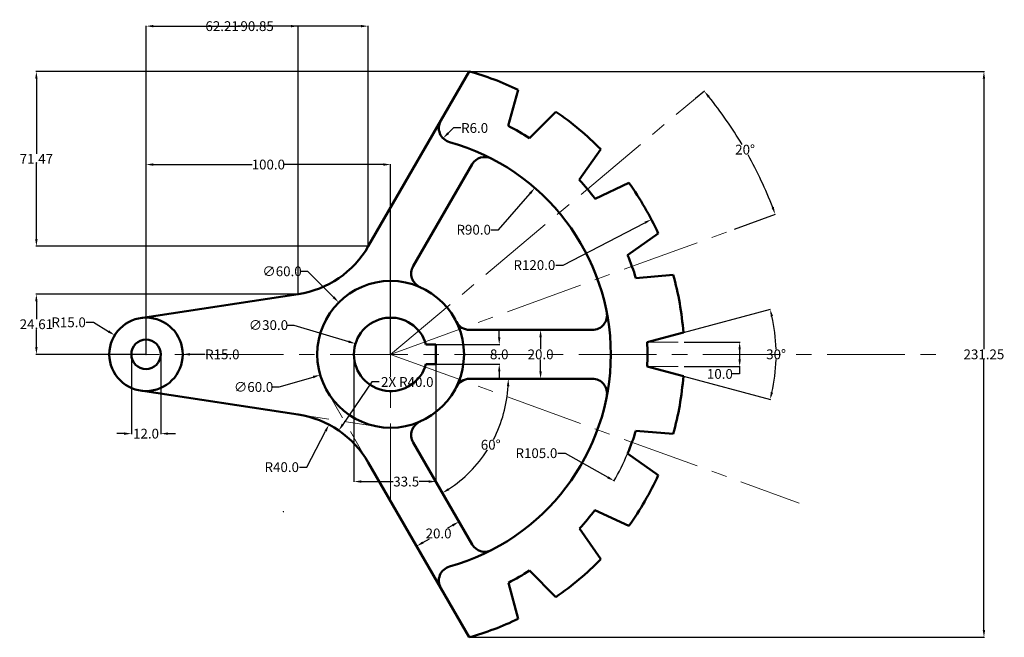
# Model space of a CAD drawing. Units: inches. Extents: x 327 to 730, y 258 to 510.
import ezdxf

# ---------------------------------------------------------------- set-up
doc = ezdxf.new("R2010")
doc.units = ezdxf.units.IN
doc.header["$MEASUREMENT"] = 0
doc.linetypes.add('CENTER', pattern=[50.8, 31.75, -6.35, 6.35, -6.35])
doc.linetypes.add('DASHED', pattern=[19.05, 12.7, -6.35])
for name, color, linetype, lineweight in [('M-CNTR', 4, 'CENTER', 18), ('M-CONS', 8, 'DASHED', 13), ('M-DIMS', 2, 'Continuous', 25), ('M-OUTL', 7, 'Continuous', 50)]:
    doc.layers.add(name, color=color, linetype=linetype, lineweight=lineweight)
doc.styles.get("Standard").update_dxf_attribs({"font": 'arial.ttf'})
doc.dimstyles.get("Standard").update_dxf_attribs({"dimtxt": 4, "dimasz": 3, "dimexe": 0.18, "dimexo": 0.0625, "dimgap": 0.09, "dimtad": 0, "dimtih": 1, "dimtoh": 1, "dimdec": 1, "dimzin": 0, "dimdsep": 46, "dimtxsty": 'Standard', "dimcen": 0.09, "dimadec": 0, "dimazin": 0, "dimtfac": 1, "dimtdec": 1, "dimtofl": 0, "dimtmove": 0, "dimatfit": 3, "dimfxl": 1, "dimtolj": 1, "dimtzin": 0, "dimarcsym": 0})

# ---------------------------------------------------------------- blocks, each defined once
blk = doc.blocks.new('*D1')
at = {"layer": 'Defpoints', "color": 0, "transparency": 16777216}
for p in [(463.65, 373.45), (497.15, 373.45), (497.15, 321.47)]:
    blk.add_point(p, dxfattribs=at)
at = {"layer": 'M-DIMS', "color": 0, "lineweight": -2, "transparency": 16777216}
for p, q in [((463.65, 373.39), (463.65, 321.29)), ((497.15, 373.39), (497.15, 321.29)), ((466.65, 321.47), (479.73, 321.47)), ((494.15, 321.47), (490.33, 321.47))]:
    blk.add_line(p, q, dxfattribs=at)
at = {"layer": 'M-DIMS', "color": 0, "transparency": 16777216}
for points in [[(466.65, 321.97), (466.65, 320.97), (463.65, 321.47)], [(494.15, 321.97), (494.15, 320.97), (497.15, 321.47)]]:
    blk.add_solid(points, dxfattribs=at)
at = {"layer": 'M-DIMS', "color": 0, "transparency": 16777216, "insert": (485.03, 321.47), "char_height": 4, "attachment_point": 5}
blk.add_mtext('\\A1;33.5', dxfattribs=at)
blk = doc.blocks.new('*D2')
at = {"layer": 'Defpoints', "color": 0, "transparency": 16777216}
for p in [(497.15, 377.45), (497.15, 369.45), (523.04, 369.45)]:
    blk.add_point(p, dxfattribs=at)
at = {"layer": 'M-DIMS', "color": 0, "lineweight": -2, "transparency": 16777216}
for p, q in [((523.04, 380.45), (523.04, 383.45)), ((497.21, 377.45), (523.22, 377.45)), ((497.21, 369.45), (523.22, 369.45)), ((523.04, 366.45), (523.04, 363.45))]:
    blk.add_line(p, q, dxfattribs=at)
at = {"layer": 'M-DIMS', "color": 0, "transparency": 16777216}
for points in [[(522.54, 380.45), (523.54, 380.45), (523.04, 377.45)], [(522.54, 366.45), (523.54, 366.45), (523.04, 369.45)]]:
    blk.add_solid(points, dxfattribs=at)
at = {"layer": 'M-DIMS', "color": 0, "transparency": 16777216, "insert": (523.04, 373.45), "char_height": 4, "attachment_point": 5}
blk.add_mtext('\\A1;8.0', dxfattribs=at)
blk = doc.blocks.new('*D3')
at = {"layer": 'Defpoints', "color": 0, "transparency": 16777216}
for p in [(539.95, 383.45), (539.95, 363.45), (539.95, 363.45)]:
    blk.add_point(p, dxfattribs=at)
at = {"layer": 'M-DIMS', "color": 0, "lineweight": -2, "transparency": 16777216}
for p, q in [((540.01, 383.45), (540.13, 383.45)), ((539.95, 380.45), (539.95, 375.58)), ((539.95, 366.45), (539.95, 371.32)), ((540.01, 363.45), (540.13, 363.45))]:
    blk.add_line(p, q, dxfattribs=at)
at = {"layer": 'M-DIMS', "color": 0, "transparency": 16777216}
for points in [[(539.45, 380.45), (540.45, 380.45), (539.95, 383.45)], [(539.45, 366.45), (540.45, 366.45), (539.95, 363.45)]]:
    blk.add_solid(points, dxfattribs=at)
at = {"layer": 'M-DIMS', "color": 0, "transparency": 16777216, "insert": (539.95, 373.45), "char_height": 4, "attachment_point": 5}
blk.add_mtext('\\A1;20.0', dxfattribs=at)
blk = doc.blocks.new('*D4')
at = {"layer": 'Defpoints', "color": 0, "transparency": 16777216}
for p in [(365.84, 381.27), (378.65, 373.45)]:
    blk.add_point(p, dxfattribs=at)
at = {"layer": 'M-DIMS', "color": 0, "lineweight": -2, "transparency": 16777216}
for p, q in [((354.21, 386.54), (357.21, 386.54)), ((357.21, 386.54), (363.28, 382.83)), ((378.56, 373.45), (378.74, 373.45)), ((378.65, 373.36), (378.65, 373.54))]:
    blk.add_line(p, q, dxfattribs=at)
at = {"layer": 'M-DIMS', "color": 0, "transparency": 16777216}
blk.add_solid([(363.54, 383.26), (363.02, 382.4), (365.84, 381.27)], dxfattribs=at)
at = {"layer": 'M-DIMS', "color": 0, "transparency": 16777216, "insert": (347.01, 386.54), "char_height": 4, "attachment_point": 5}
blk.add_mtext('\\A1;R15.0', dxfattribs=at)
blk = doc.blocks.new('*D5')
at = {"layer": 'Defpoints', "color": 0, "transparency": 16777216}
for p in [(372.65, 373.45), (384.65, 373.45), (384.65, 341.05)]:
    blk.add_point(p, dxfattribs=at)
at = {"layer": 'M-DIMS', "color": 0, "lineweight": -2, "transparency": 16777216}
for p, q in [((372.65, 373.39), (372.65, 340.87)), ((384.65, 373.39), (384.65, 340.87)), ((369.65, 341.05), (366.65, 341.05)), ((387.65, 341.05), (390.65, 341.05))]:
    blk.add_line(p, q, dxfattribs=at)
at = {"layer": 'M-DIMS', "color": 0, "transparency": 16777216}
for points in [[(369.65, 341.55), (369.65, 340.55), (372.65, 341.05)], [(387.65, 341.55), (387.65, 340.55), (384.65, 341.05)]]:
    blk.add_solid(points, dxfattribs=at)
at = {"layer": 'M-DIMS', "color": 0, "transparency": 16777216, "insert": (378.65, 341.05), "char_height": 4, "attachment_point": 5}
blk.add_mtext('\\A1;12.0', dxfattribs=at)
blk = doc.blocks.new('*D6')
at = {"layer": 'Defpoints', "color": 0, "transparency": 16777216}
for p in [(507.44, 381.88), (449.85, 365.03)]:
    blk.add_point(p, dxfattribs=at)
at = {"layer": 'M-DIMS', "color": 0, "lineweight": -2, "transparency": 16777216}
for p, q in [((478.56, 373.45), (478.74, 373.45)), ((478.65, 373.36), (478.65, 373.54)), ((433.09, 360.12), (446.97, 364.18)), ((430.09, 360.12), (433.09, 360.12))]:
    blk.add_line(p, q, dxfattribs=at)
at = {"layer": 'M-DIMS', "color": 0, "transparency": 16777216}
blk.add_solid([(446.83, 364.66), (447.11, 363.7), (449.85, 365.03)], dxfattribs=at)
at = {"layer": 'M-DIMS', "color": 0, "transparency": 16777216, "insert": (422.63, 360.12), "char_height": 4, "attachment_point": 5}
blk.add_mtext('\\A1;∅60.0', dxfattribs=at)
blk = doc.blocks.new('*D7')
at = {"layer": 'Defpoints', "color": 0, "transparency": 16777216}
for p in [(464.29, 377.8), (493, 369.11)]:
    blk.add_point(p, dxfattribs=at)
at = {"layer": 'M-DIMS', "color": 0, "lineweight": -2, "transparency": 16777216}
for p, q in [((436.14, 385.4), (439.14, 385.4)), ((439.14, 385.4), (461.42, 378.66)), ((478.56, 373.45), (478.74, 373.45)), ((478.65, 373.36), (478.65, 373.54))]:
    blk.add_line(p, q, dxfattribs=at)
at = {"layer": 'M-DIMS', "color": 0, "transparency": 16777216}
blk.add_solid([(461.56, 379.14), (461.27, 378.19), (464.29, 377.8)], dxfattribs=at)
at = {"layer": 'M-DIMS', "color": 0, "transparency": 16777216, "insert": (428.69, 385.4), "char_height": 4, "attachment_point": 5}
blk.add_mtext('\\A1;∅30.0', dxfattribs=at)
blk = doc.blocks.new('*D8')
at = {"layer": 'Defpoints', "color": 0, "transparency": 16777216}
for p in [(500.21, 316.1), (482.89, 306.1), (489.26, 295.07)]:
    blk.add_point(p, dxfattribs=at)
at = {"layer": 'M-DIMS', "color": 0, "lineweight": -2, "transparency": 16777216}
for p, q in [((500.24, 316.05), (506.67, 304.91)), ((482.92, 306.05), (489.35, 294.91)), ((503.98, 303.57), (501.94, 302.39)), ((491.86, 296.57), (494.55, 298.12))]:
    blk.add_line(p, q, dxfattribs=at)
at = {"layer": 'M-DIMS', "color": 0, "transparency": 16777216}
for points in [[(503.73, 304), (504.23, 303.14), (506.58, 305.07)], [(491.61, 297), (492.11, 296.14), (489.26, 295.07)]]:
    blk.add_solid(points, dxfattribs=at)
at = {"layer": 'M-DIMS', "color": 0, "transparency": 16777216, "insert": (498.25, 300.26), "char_height": 4, "attachment_point": 5}
blk.add_mtext('\\A1;20.0', dxfattribs=at)
blk = doc.blocks.new('*D9')
at = {"layer": 'Defpoints', "color": 0, "transparency": 16777216}
for p in [(598.54, 378.45), (598.54, 368.45), (621.33, 368.45)]:
    blk.add_point(p, dxfattribs=at)
at = {"layer": 'M-DIMS', "color": 0, "lineweight": -2, "transparency": 16777216}
for p, q in [((598.6, 378.45), (621.51, 378.45)), ((621.33, 375.45), (621.33, 371.45)), ((598.6, 368.45), (621.51, 368.45)), ((621.33, 368.45), (621.33, 365.45)), ((621.33, 365.45), (618.33, 365.45))]:
    blk.add_line(p, q, dxfattribs=at)
at = {"layer": 'M-DIMS', "color": 0, "transparency": 16777216}
for points in [[(620.83, 375.45), (621.83, 375.45), (621.33, 378.45)], [(620.83, 371.45), (621.83, 371.45), (621.33, 368.45)]]:
    blk.add_solid(points, dxfattribs=at)
at = {"layer": 'M-DIMS', "color": 0, "transparency": 16777216, "insert": (613.24, 365.45), "char_height": 4, "attachment_point": 5}
blk.add_mtext('\\A1;10.0', dxfattribs=at)
blk = doc.blocks.new('*D10')
at = {"layer": 'Defpoints', "color": 0, "transparency": 16777216}
for p in [(598.31, 382.41), (583.53, 378.45), (583.53, 368.45), (635.95, 367.23), (598.31, 364.49)]:
    blk.add_point(p, dxfattribs=at)
at = {"layer": 'M-DIMS', "color": 0, "lineweight": -2, "transparency": 16777216}
for p, q in [((598.37, 382.43), (633.96, 391.97)), ((598.37, 364.47), (633.96, 354.94))]:
    blk.add_line(p, q, dxfattribs=at)
for start, end in [(1.7136, 12.5908), (347.4092, 358.2864)]:
    blk.add_arc((564.87, 373.45), 71.35, start, end, dxfattribs=at)
at = {"layer": 'M-DIMS', "color": 0, "transparency": 16777216}
for points in [[(634.02, 388.89), (634.99, 389.12), (633.79, 391.92)], [(634.99, 357.78), (634.02, 358.02), (633.79, 354.98)]]:
    blk.add_solid(points, dxfattribs=at)
at = {"layer": 'M-DIMS', "color": 0, "transparency": 16777216, "insert": (636.22, 373.45), "char_height": 4, "attachment_point": 5}
blk.add_mtext('\\A1;30°', dxfattribs=at)
blk = doc.blocks.new('*U11')
for p, q in [((-7.39, 5), (7.39, 8.96)), ((-7.39, -5), (7.39, -8.96))]:
    blk.add_line(p, q)
blk.add_arc((-112.27, 0), 105, 357.2706, 2.7294)
blk = doc.blocks.new('*U12')
at = {"layer": 'M-OUTL', "color": 0, "linetype": 'ByBlock', "lineweight": -2, "transparency": 16777216}
for p, rotation in [((534.78, 470.68), 59.99999999999994), ((564.65, 445.62), 39.99999999999997), ((584.15, 411.85), 19.99999999999995)]:
    blk.add_blockref('*U11', p, dxfattribs=dict(at, rotation=rotation))
blk.add_blockref('*U11', (590.92, 373.45), dxfattribs=at)
blk = doc.blocks.new('*D13')
at = {"layer": 'Defpoints', "color": 0, "transparency": 16777216}
for p in [(603.28, 478.03), (628.17, 448.54), (619.17, 424.6), (478.65, 373.45), (478.65, 373.45)]:
    blk.add_point(p, dxfattribs=at)
at = {"layer": 'M-DIMS', "color": 0, "lineweight": -2, "transparency": 16777216}
for p, q in [((603.33, 478.07), (606.96, 481.12)), ((619.23, 424.62), (636.04, 430.74))]:
    blk.add_line(p, q, dxfattribs=at)
for start, end in [(30.8468, 38.9727), (21.0273, 29.1604)]:
    blk.add_arc((478.65, 373.45), 167.32, start, end, dxfattribs=at)
at = {"layer": 'M-DIMS', "color": 0, "transparency": 16777216}
for points in [[(608.34, 478.37), (609.11, 479), (606.82, 481)], [(635.29, 433.66), (634.35, 433.31), (635.87, 430.68)]]:
    blk.add_solid(points, dxfattribs=at)
at = {"layer": 'M-DIMS', "color": 0, "transparency": 16777216, "insert": (623.55, 457.11), "char_height": 4, "attachment_point": 5}
blk.add_mtext('\\A1;20°', dxfattribs=at)
blk = doc.blocks.new('*D14')
at = {"layer": 'Defpoints', "color": 0, "transparency": 16777216}
for p in [(453.44, 344.72), (434.86, 309.29)]:
    blk.add_point(p, dxfattribs=at)
at = {"layer": 'M-DIMS', "color": 0, "lineweight": -2, "transparency": 16777216}
for p, q in [((444.34, 327.36), (452.05, 342.06)), ((441.34, 327.36), (444.34, 327.36))]:
    blk.add_line(p, q, dxfattribs=at)
at = {"layer": 'M-DIMS', "color": 0, "transparency": 16777216}
blk.add_solid([(451.6, 342.29), (452.49, 341.83), (453.44, 344.72)], dxfattribs=at)
at = {"layer": 'M-DIMS', "color": 0, "transparency": 16777216, "insert": (434.14, 327.36), "char_height": 4, "attachment_point": 5}
blk.add_mtext('\\A1;R40.0', dxfattribs=at)
blk = doc.blocks.new('*D15')
at = {"layer": 'Defpoints', "color": 0, "transparency": 16777216}
for p in [(478.65, 373.45), (570.03, 321.73)]:
    blk.add_point(p, dxfattribs=at)
at = {"layer": 'M-DIMS', "color": 0, "lineweight": -2, "transparency": 16777216}
for p, q in [((547, 333.07), (550, 333.07)), ((550, 333.07), (567.41, 323.21))]:
    blk.add_line(p, q, dxfattribs=at)
blk.add_arc((478.65, 373.45), 105, 330.3928, 337.2537, dxfattribs=at)
at = {"layer": 'M-DIMS', "color": 0, "transparency": 16777216}
blk.add_solid([(567.66, 323.65), (567.17, 322.77), (570.03, 321.73)], dxfattribs=at)
at = {"layer": 'M-DIMS', "color": 0, "transparency": 16777216, "insert": (538.25, 333.07), "char_height": 4, "attachment_point": 5}
blk.add_mtext('\\A1;R105.0', dxfattribs=at)
blk = doc.blocks.new('*U16')
for p, q in [((-5.92, 9.06), (9.32, 7.72)), ((-9.32, -0.28), (3.21, -9.06))]:
    blk.add_line(p, q)
blk.add_arc((-106.18, 40.26), 105, 337.2878, 342.7122)
blk = doc.blocks.new('*U17')
at = {"layer": 'M-OUTL', "color": 0, "linetype": 'ByBlock', "lineweight": -2, "transparency": 16777216}
blk.add_blockref('*U16', (584.83, 333.19), dxfattribs=at)
for p, rotation in [((564.65, 299.3), 340.0000000000001), ((534.11, 274.36), 320.0000000000001)]:
    blk.add_blockref('*U16', p, dxfattribs=dict(at, rotation=rotation))
blk = doc.blocks.new('*D18')
at = {"layer": 'Defpoints', "color": 0, "transparency": 16777216}
for p in [(537.6, 441.46), (478.65, 373.45)]:
    blk.add_point(p, dxfattribs=at)
at = {"layer": 'M-DIMS', "color": 0, "lineweight": -2, "transparency": 16777216}
for p, q in [((522.8, 424.38), (535.63, 439.19)), ((519.8, 424.38), (522.8, 424.38))]:
    blk.add_line(p, q, dxfattribs=at)
at = {"layer": 'M-DIMS', "color": 0, "transparency": 16777216}
blk.add_solid([(535.26, 439.52), (536.01, 438.86), (537.6, 441.46)], dxfattribs=at)
at = {"layer": 'M-DIMS', "color": 0, "transparency": 16777216, "insert": (512.61, 424.38), "char_height": 4, "attachment_point": 5}
blk.add_mtext('\\A1;R90.0', dxfattribs=at)
blk = doc.blocks.new('*D19')
at = {"layer": 'Defpoints', "color": 0, "transparency": 16777216}
for p in [(585.23, 428.58), (478.65, 373.45)]:
    blk.add_point(p, dxfattribs=at)
at = {"layer": 'M-DIMS', "color": 0, "lineweight": -2, "transparency": 16777216}
for p, q in [((549.17, 409.92), (582.57, 427.2)), ((546.17, 409.92), (549.17, 409.92))]:
    blk.add_line(p, q, dxfattribs=at)
at = {"layer": 'M-DIMS', "color": 0, "transparency": 16777216}
blk.add_solid([(582.34, 427.64), (582.8, 426.76), (585.23, 428.58)], dxfattribs=at)
at = {"layer": 'M-DIMS', "color": 0, "transparency": 16777216, "insert": (537.42, 409.92), "char_height": 4, "attachment_point": 5}
blk.add_mtext('\\A1;R120.0', dxfattribs=at)
blk = doc.blocks.new('*D20')
at = {"layer": 'Defpoints', "color": 0, "transparency": 16777216}
for p in [(378.65, 451.01), (378.65, 373.45), (478.65, 373.45)]:
    blk.add_point(p, dxfattribs=at)
at = {"layer": 'M-DIMS', "color": 0, "lineweight": -2, "transparency": 16777216}
for p, q in [((378.65, 373.51), (378.65, 451.19)), ((381.65, 451.01), (422, 451.01)), ((475.65, 451.01), (435.29, 451.01)), ((478.65, 373.51), (478.65, 451.19))]:
    blk.add_line(p, q, dxfattribs=at)
at = {"layer": 'M-DIMS', "color": 0, "transparency": 16777216}
for points in [[(381.65, 451.51), (381.65, 450.51), (378.65, 451.01)], [(475.65, 451.51), (475.65, 450.51), (478.65, 451.01)]]:
    blk.add_solid(points, dxfattribs=at)
at = {"layer": 'M-DIMS', "color": 0, "transparency": 16777216, "insert": (428.65, 451.01), "char_height": 4, "attachment_point": 5}
blk.add_mtext('\\A1;100.0', dxfattribs=at)
blk = doc.blocks.new('*D21')
at = {"layer": 'Defpoints', "color": 0, "transparency": 16777216}
for p in [(504.34, 465.95), (500.05, 461.75)]:
    blk.add_point(p, dxfattribs=at)
at = {"layer": 'M-DIMS', "color": 0, "lineweight": -2, "transparency": 16777216}
for p, q in [((504.34, 465.95), (502.2, 463.85)), ((507.34, 465.95), (504.34, 465.95))]:
    blk.add_line(p, q, dxfattribs=at)
at = {"layer": 'M-DIMS', "color": 0, "transparency": 16777216}
blk.add_solid([(501.85, 464.21), (502.55, 463.49), (500.05, 461.75)], dxfattribs=at)
at = {"layer": 'M-DIMS', "color": 0, "transparency": 16777216, "insert": (512.98, 465.95), "char_height": 4, "attachment_point": 5}
blk.add_mtext('\\A1;R6.0', dxfattribs=at)
blk = doc.blocks.new('*D22')
at = {"layer": 'Defpoints', "color": 0, "transparency": 16777216}
for p in [(510.9, 363.45), (561.11, 363.45), (487.87, 337.47), (514.15, 328.82), (511.94, 295.79)]:
    blk.add_point(p, dxfattribs=at)
at = {"layer": 'M-DIMS', "color": 0, "lineweight": -2, "transparency": 16777216}
for start, end in [(332.5853, 356.8096), (303.1904, 327.3455)]:
    blk.add_arc((472.87, 363.45), 53.88, start, end, dxfattribs=at)
at = {"layer": 'M-DIMS', "color": 0, "transparency": 16777216}
for points in [[(526.17, 360.47), (527.17, 360.44), (526.76, 363.45)], [(502.63, 317.93), (502.11, 318.78), (499.81, 316.79)]]:
    blk.add_solid(points, dxfattribs=at)
at = {"layer": 'M-DIMS', "color": 0, "transparency": 16777216, "insert": (519.54, 336.51), "char_height": 4, "attachment_point": 5}
blk.add_mtext('\\A1;60°', dxfattribs=at)
blk = doc.blocks.new('*D23')
at = {"layer": 'Defpoints', "color": 0, "transparency": 16777216}
for p in [(510.76, 489.07), (510.76, 257.83), (721.19, 257.83)]:
    blk.add_point(p, dxfattribs=at)
at = {"layer": 'M-DIMS', "color": 0, "lineweight": -2, "transparency": 16777216}
for p, q in [((510.82, 489.07), (721.37, 489.07)), ((721.19, 486.07), (721.19, 375.58)), ((721.19, 260.83), (721.19, 371.32)), ((510.82, 257.83), (721.37, 257.83))]:
    blk.add_line(p, q, dxfattribs=at)
at = {"layer": 'M-DIMS', "color": 0, "transparency": 16777216}
for points in [[(720.69, 486.07), (721.69, 486.07), (721.19, 489.07)], [(720.69, 260.83), (721.69, 260.83), (721.19, 257.83)]]:
    blk.add_solid(points, dxfattribs=at)
at = {"layer": 'M-DIMS', "color": 0, "transparency": 16777216, "insert": (721.19, 373.45), "char_height": 4, "attachment_point": 5}
blk.add_mtext('\\A1;231.25', dxfattribs=at)
blk = doc.blocks.new('*D24')
at = {"layer": 'Defpoints', "color": 0, "transparency": 16777216}
for p in [(333.82, 398.06), (440.86, 398.06), (378.65, 373.45)]:
    blk.add_point(p, dxfattribs=at)
at = {"layer": 'M-DIMS', "color": 0, "lineweight": -2, "transparency": 16777216}
for p, q in [((440.8, 398.06), (333.64, 398.06)), ((333.82, 395.06), (333.82, 387.89)), ((333.82, 376.45), (333.82, 383.62)), ((378.58, 373.45), (333.64, 373.45))]:
    blk.add_line(p, q, dxfattribs=at)
at = {"layer": 'M-DIMS', "color": 0, "transparency": 16777216}
for points in [[(333.32, 395.06), (334.32, 395.06), (333.82, 398.06)], [(333.32, 376.45), (334.32, 376.45), (333.82, 373.45)]]:
    blk.add_solid(points, dxfattribs=at)
at = {"layer": 'M-DIMS', "color": 0, "transparency": 16777216, "insert": (333.82, 385.76), "char_height": 4, "attachment_point": 5}
blk.add_mtext('\\A1;24.61', dxfattribs=at)
blk = doc.blocks.new('*D25')
at = {"layer": 'Defpoints', "color": 0, "transparency": 16777216}
for p in [(440.86, 507.57), (440.86, 398.06), (378.65, 373.45)]:
    blk.add_point(p, dxfattribs=at)
at = {"layer": 'M-DIMS', "color": 0, "lineweight": -2, "transparency": 16777216}
for p, q in [((378.65, 373.51), (378.65, 507.75)), ((381.65, 507.57), (403.29, 507.57)), ((437.86, 507.57), (416.22, 507.57)), ((440.86, 398.12), (440.86, 507.75))]:
    blk.add_line(p, q, dxfattribs=at)
at = {"layer": 'M-DIMS', "color": 0, "transparency": 16777216}
for points in [[(381.65, 508.07), (381.65, 507.07), (378.65, 507.57)], [(437.86, 508.07), (437.86, 507.07), (440.86, 507.57)]]:
    blk.add_solid(points, dxfattribs=at)
at = {"layer": 'M-DIMS', "color": 0, "transparency": 16777216, "insert": (409.75, 507.57), "char_height": 4, "attachment_point": 5}
blk.add_mtext('\\A1;62.21', dxfattribs=at)
blk = doc.blocks.new('*D26')
at = {"layer": 'Defpoints', "color": 0, "transparency": 16777216}
for p in [(333.82, 489.07), (510.76, 489.07), (469.5, 417.61)]:
    blk.add_point(p, dxfattribs=at)
at = {"layer": 'M-DIMS', "color": 0, "lineweight": -2, "transparency": 16777216}
for p, q in [((510.7, 489.07), (333.64, 489.07)), ((333.82, 486.07), (333.82, 455.44)), ((333.82, 420.61), (333.82, 451.24)), ((469.44, 417.61), (333.64, 417.61))]:
    blk.add_line(p, q, dxfattribs=at)
at = {"layer": 'M-DIMS', "color": 0, "transparency": 16777216}
for points in [[(333.32, 486.07), (334.32, 486.07), (333.82, 489.07)], [(333.32, 420.61), (334.32, 420.61), (333.82, 417.61)]]:
    blk.add_solid(points, dxfattribs=at)
at = {"layer": 'M-DIMS', "color": 0, "transparency": 16777216, "insert": (333.82, 453.34), "char_height": 4, "attachment_point": 5}
blk.add_mtext('\\A1;71.47', dxfattribs=at)
blk = doc.blocks.new('*D27')
at = {"layer": 'Defpoints', "color": 0, "transparency": 16777216}
for p in [(469.5, 507.57), (469.5, 417.61), (378.65, 373.45)]:
    blk.add_point(p, dxfattribs=at)
at = {"layer": 'M-DIMS', "color": 0, "lineweight": -2, "transparency": 16777216}
for p, q in [((378.65, 373.51), (378.65, 507.75)), ((381.65, 507.57), (417.22, 507.57)), ((466.5, 507.57), (430.93, 507.57)), ((469.5, 417.67), (469.5, 507.75))]:
    blk.add_line(p, q, dxfattribs=at)
at = {"layer": 'M-DIMS', "color": 0, "transparency": 16777216}
for points in [[(381.65, 508.07), (381.65, 507.07), (378.65, 507.57)], [(466.5, 508.07), (466.5, 507.07), (469.5, 507.57)]]:
    blk.add_solid(points, dxfattribs=at)
at = {"layer": 'M-DIMS', "color": 0, "transparency": 16777216, "insert": (424.07, 507.57), "char_height": 4, "attachment_point": 5}
blk.add_mtext('\\A1;90.85', dxfattribs=at)
blk = doc.blocks.new('*D28')
at = {"layer": 'Defpoints', "color": 0, "transparency": 16777216}
for p in [(457.41, 342.33), (434.86, 309.29)]:
    blk.add_point(p, dxfattribs=at)
at = {"layer": 'M-DIMS', "color": 0, "lineweight": -2, "transparency": 16777216}
for p, q in [((470.94, 362.16), (459.1, 344.81)), ((473.94, 362.16), (470.94, 362.16)), ((434.77, 309.29), (434.95, 309.29)), ((434.86, 309.2), (434.86, 309.38))]:
    blk.add_line(p, q, dxfattribs=at)
at = {"layer": 'M-DIMS', "color": 0, "transparency": 16777216}
blk.add_solid([(458.69, 345.09), (459.51, 344.53), (457.41, 342.33)], dxfattribs=at)
at = {"layer": 'M-DIMS', "color": 0, "transparency": 16777216, "insert": (485.46, 362.16), "char_height": 4, "attachment_point": 5}
blk.add_mtext('\\A1;2X R40.0', dxfattribs=at)
blk = doc.blocks.new('*D29')
at = {"layer": 'Defpoints', "color": 0, "transparency": 16777216}
for p in [(457.43, 394.67), (499.86, 352.24)]:
    blk.add_point(p, dxfattribs=at)
at = {"layer": 'M-DIMS', "color": 0, "lineweight": -2, "transparency": 16777216}
for p, q in [((441.71, 407.39), (444.71, 407.39)), ((444.71, 407.39), (455.31, 396.79)), ((478.56, 373.45), (478.74, 373.45)), ((478.65, 373.36), (478.65, 373.54))]:
    blk.add_line(p, q, dxfattribs=at)
at = {"layer": 'M-DIMS', "color": 0, "transparency": 16777216}
blk.add_solid([(455.67, 397.14), (454.96, 396.43), (457.43, 394.67)], dxfattribs=at)
at = {"layer": 'M-DIMS', "color": 0, "transparency": 16777216, "insert": (434.25, 407.39), "char_height": 4, "attachment_point": 5}
blk.add_mtext('\\A1;∅60.0', dxfattribs=at)
blk = doc.blocks.new('*D30')
at = {"layer": 'Defpoints', "color": 0, "transparency": 16777216}
for p in [(378.65, 373.45), (393.65, 373.45)]:
    blk.add_point(p, dxfattribs=at)
at = {"layer": 'M-DIMS', "color": 0, "lineweight": -2, "transparency": 16777216}
for p, q in [((378.56, 373.45), (378.74, 373.45)), ((378.65, 373.36), (378.65, 373.54)), ((402.65, 373.45), (396.65, 373.45))]:
    blk.add_line(p, q, dxfattribs=at)
at = {"layer": 'M-DIMS', "color": 0, "transparency": 16777216}
blk.add_solid([(396.65, 373.95), (396.65, 372.95), (393.65, 373.45)], dxfattribs=at)
at = {"layer": 'M-DIMS', "color": 0, "transparency": 16777216, "insert": (409.84, 373.45), "char_height": 4, "attachment_point": 5}
blk.add_mtext('\\A1;R15.0', dxfattribs=at)

msp = doc.modelspace()

# ---------------------------------------------------------------- linework, layer by layer
at = {"layer": 'M-CNTR'}
for p, q in [((478.646, 373.451), (603.282, 478.033)), ((478.646, 373.451), (619.173, 424.599)), ((478.646, 313.451), (478.646, 403.451)), ((352.317, 373.451), (702.691, 373.451)), ((478.646, 373.451), (645.677, 312.657))]:
    msp.add_line(p, q, dxfattribs=at)
at = {"layer": 'M-CONS'}
for p, q in [((583.527, 378.451), (598.542, 378.451)), ((583.527, 368.451), (598.542, 368.451)), ((452.665, 358.451), (469.5, 329.294)), ((440.859, 348.841), (474.146, 343.791)), ((499.141, 277.953), (510.76, 257.828))]:
    msp.add_line(p, q, dxfattribs=at)
at = {"layer": 'M-OUTL'}
for p, q in [((469.5, 417.609), (510.76, 489.074)), ((487.874, 409.435), (511.938, 451.115)), ((376.396, 388.282), (440.859, 398.062)), ((510.895, 383.451), (561.108, 383.451)), ((493.103, 377.451), (497.146, 377.451)), ((497.146, 377.451), (497.146, 369.451)), ((493.103, 369.451), (497.146, 369.451)), ((510.895, 363.451), (561.108, 363.451)), ((376.396, 358.621), (440.859, 348.841)), ((487.874, 337.467), (511.938, 295.788)), ((469.5, 329.294), (510.76, 257.828))]:
    msp.add_line(p, q, dxfattribs=at)
for centre, radius in [((478.646, 373.451), 30), ((378.646, 373.451), 15), ((378.646, 373.451), 6)]:
    msp.add_circle(centre, radius, dxfattribs=at)
for centre, radius, start, end in [((478.646, 373.451), 120, 64.28273, 74.47751), ((478.646, 373.451), 120, 44.28273, 55.71727), ((504.337, 465.95), 6, 150, 254.47751), ((478.646, 373.451), 90, 285.52249, 74.47751), ((517.134, 448.115), 6, 62.7294, 150), ((478.646, 373.451), 120, 24.28273, 35.71727), ((434.859, 437.609), 40, 278.62693, 330), ((493.071, 406.435), 6, 150, 246.37937), ((478.646, 373.451), 120, 4.28273, 15.71727), ((561.108, 389.451), 6, 270, 10.98058), ((478.646, 373.451), 15, 15.46601, 344.53399), ((510.895, 389.451), 6, 206.3878, 270), ((510.895, 357.451), 6, 90, 153.6122), ((561.108, 357.451), 6, 349.01942, 90), ((478.646, 373.451), 120, 344.26774, 355.71727), ((434.859, 309.294), 40, 30, 81.37307), ((493.071, 340.467), 6, 113.62063, 210), ((478.646, 373.451), 120, 324.26774, 335.73226), ((517.134, 298.788), 6, 210, 297.2706), ((504.337, 280.953), 6, 105.52249, 210), ((478.646, 373.451), 120, 304.26774, 315.73226), ((478.646, 373.451), 120, 285.52249, 295.73226)]:
    msp.add_arc(centre, radius, start, end, dxfattribs=at)

# ---------------------------------------------------------------- block references
for name in ['*U12', '*U17']:
    msp.add_blockref(name, (0, 0), dxfattribs=at)

# ---------------------------------------------------------------- dimensions: what is measured, and where the dimension line sits
at = {"layer": 'M-DIMS'}
for base, p1, p2, override, picture, middle in [((440.859, 507.574), (378.646, 373.451), (440.859, 398.062), {"dimdec": 2, "dimlfac": 1, "dimrnd": 0, "dimzin": 0, "dimdsep": 46, "dimlunit": 2}, '*D25', (409.752, 507.574)), ((469.5, 507.574), (378.646, 373.451), (469.5, 417.609), {"dimdec": 2, "dimlfac": 1, "dimrnd": 0, "dimzin": 0, "dimdsep": 46, "dimlunit": 2}, '*D27', (424.073, 507.574)), ((378.646, 451.01), (478.646, 373.451), (378.646, 373.451), {"dimclrd": 0, "dimclre": 0, "dimclrt": 0}, '*D20', (428.646, 451.01)), ((384.646, 341.05), (372.646, 373.451), (384.646, 373.451), {"dimclrd": 0, "dimclre": 0, "dimclrt": 0}, '*D5', (378.646, 341.05))]:
    dim = msp.add_linear_dim(base=base, p1=p1, p2=p2, dimstyle='Standard', override=override, dxfattribs=at)
    dim.commit()
    dim.dimension.update_dxf_attribs({"geometry": picture, "text_midpoint": middle})
for base, p1, p2, override, picture, middle in [((333.8174, 489.0744), (469.4996, 417.6091), (510.7601, 489.0744), {"dimdec": 2, "dimlfac": 1, "dimrnd": 0, "dimzin": 0, "dimdsep": 46, "dimlunit": 2}, '*D26', (333.8174, 453.3417)), ((721.191, 257.828), (510.76, 489.074), (510.76, 257.828), {"dimdec": 2, "dimlfac": 1, "dimrnd": 0, "dimzin": 0, "dimdsep": 46, "dimlunit": 2}, '*D23', (721.191, 373.451)), ((333.817, 398.062), (378.646, 373.451), (440.859, 398.062), {"dimdec": 2, "dimlfac": 1, "dimrnd": 0, "dimzin": 0, "dimdsep": 46, "dimlunit": 2}, '*D24', (333.817, 385.756)), ((539.947, 363.451), (539.947, 383.451), (539.947, 363.451), {"dimclrd": 0, "dimclre": 0, "dimclrt": 0}, '*D3', (539.947, 373.451)), ((621.334, 368.451), (598.542, 378.451), (598.542, 368.451), {"dimclrd": 0, "dimclre": 0, "dimclrt": 0}, '*D9', (613.244, 365.451))]:
    dim = msp.add_linear_dim(base=base, p1=p1, p2=p2, angle=90, dimstyle='Standard', override=override, dxfattribs=at)
    dim.commit()
    dim.dimension.update_dxf_attribs({"geometry": picture, "text_midpoint": middle})
for base, line1, line2, picture, middle in [((628.166, 448.543), ((478.646, 373.451), (619.173, 424.599)), ((478.646, 373.451), (603.282, 478.033)), '*D13', (623.547, 457.11)), ((635.948, 367.233), ((583.527, 368.451), (598.311, 364.49)), ((583.527, 378.451), (598.311, 382.413)), '*D10', (636.219, 373.451)), ((514.149, 328.816), ((487.874, 337.467), (511.938, 295.788)), ((510.895, 363.451), (561.108, 363.451)), '*D22', (519.537, 336.51))]:
    dim = msp.add_angular_dim_2l(base=base, line1=line1, line2=line2, dimstyle='Standard', override={"dimclrd": 0, "dimclre": 0, "dimclrt": 0}, dxfattribs=at)
    dim.commit()
    dim.dimension.update_dxf_attribs({"geometry": picture, "text_midpoint": middle})
for center, mpoint, override, picture, middle in [((504.337, 465.95), (500.053, 461.749), {"dimclrd": 0, "dimclre": 0, "dimclrt": 0}, '*D21', (512.976, 465.95)), ((478.646, 373.451), (537.599, 441.455), {"dimclrd": 0, "dimclre": 0, "dimclrt": 0}, '*D18', (512.606, 424.382)), ((478.646, 373.451), (585.234, 428.578), {"dimclrd": 0, "dimclre": 0, "dimclrt": 0}, '*D19', (537.421, 409.924)), ((378.646, 373.451), (365.843, 381.267), {"dimclrd": 0, "dimclre": 0, "dimclrt": 0}, '*D4', (347.013, 386.539)), ((378.646, 373.451), (393.646, 373.451), {"dimdec": 1, "dimlfac": 1, "dimrnd": 0, "dimzin": 0, "dimdsep": 46, "dimlunit": 2}, '*D30', (402.646, 373.451)), ((478.646, 373.451), (570.025, 321.732), {"dimclrd": 0, "dimclre": 0, "dimclrt": 0}, '*D15', (538.252, 333.067)), ((434.859, 309.294), (453.439, 344.716), {"dimclrd": 0, "dimclre": 0, "dimclrt": 0}, '*D14', (434.145, 327.365))]:
    dim = msp.add_radius_dim(center=center, mpoint=mpoint, dimstyle='Standard', override=override, dxfattribs=at)
    dim.commit()
    dim.dimension.update_dxf_attribs({"geometry": picture, "text_midpoint": middle, "dimtype": 164})
for p1, p2, override, picture, middle in [((499.858, 352.237), (457.434, 394.666), {"dimdec": 1, "dimlfac": 1, "dimrnd": 0, "dimzin": 0, "dimdsep": 46, "dimlunit": 2}, '*D29', (434.253, 407.395)), ((493.003, 369.107), (464.289, 377.795), {"dimclrd": 0, "dimclre": 0, "dimclrt": 0}, '*D7', (428.689, 385.403)), ((507.439, 381.877), (449.854, 365.026), {"dimclrd": 0, "dimclre": 0, "dimclrt": 0}, '*D6', (422.632, 360.119))]:
    dim = msp.add_diameter_dim_2p(p1=p1, p2=p2, dimstyle='Standard', override=override, dxfattribs=at)
    dim.commit()
    dim.dimension.update_dxf_attribs({"geometry": picture, "text_midpoint": middle, "dimtype": 163})
for base, p1, p2, angle, picture, middle in [((523.037, 369.451), (497.146, 377.451), (497.146, 369.451), 90, '*D2', (523.037, 373.451)), ((489.26, 295.068), (500.208, 316.104), (482.888, 306.104), 30, '*D8', (498.247, 300.257))]:
    dim = msp.add_linear_dim(base=base, p1=p1, p2=p2, angle=angle, dimstyle='Standard', override={"dimclrd": 0, "dimclre": 0, "dimclrt": 0}, dxfattribs=at)
    dim.commit()
    dim.dimension.update_dxf_attribs({"geometry": picture, "text_midpoint": middle, "dimtype": 160})
dim = msp.add_linear_dim(base=(497.146, 321.47), p1=(463.646, 373.451), p2=(497.146, 373.451), dimstyle='Standard', override={"dimclrd": 0, "dimclre": 0, "dimclrt": 0}, dxfattribs=at)
dim.commit()
dim.dimension.update_dxf_attribs({"geometry": '*D1', "text_midpoint": (485.032, 321.47), "dimtype": 160})
dim = msp.add_radius_dim(center=(434.859, 309.294), mpoint=(457.407, 342.332), text='2X <>', dimstyle='Standard', override={"dimdec": 1, "dimlfac": 1, "dimrnd": 0, "dimzin": 0, "dimdsep": 46, "dimlunit": 2}, dxfattribs=at)
dim.commit()
dim.dimension.update_dxf_attribs({"geometry": '*D28', "text_midpoint": (485.46, 362.156), "dimtype": 164})

doc.saveas('drawing.dxf')
